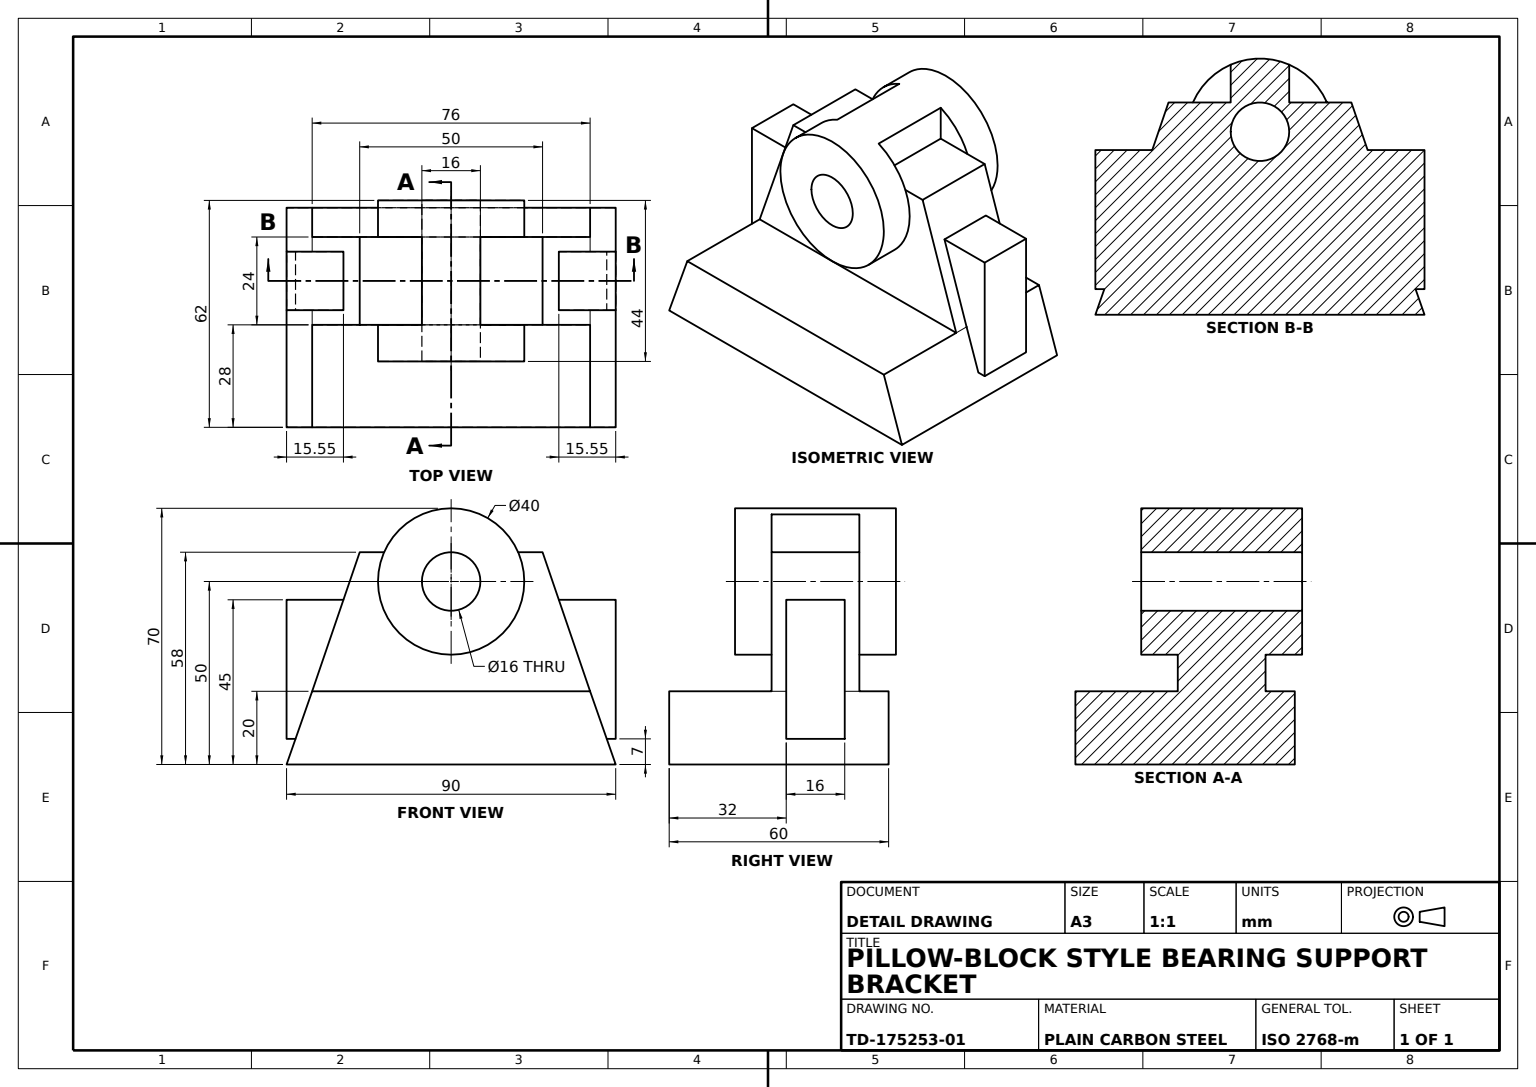
SolidWorks part; units mm, degrees
material "Plain Carbon Steel"
ref_plane "Front Plane" through (0, 0, 0) normal (0, 0, 1) x (1, 0, 0)
ref_plane "Top Plane" through (0, 0, 0) normal (0, 1, 0) x (1, 0, 0)
ref_plane "Right Plane" through (0, 0, 0) normal (1, 0, 0) x (0, 0, -1)
sketch "Base Profile Sketch" plane through (0, 0, 0) normal (0, 1, 0) x (1, 0, 0)
  line L1 (30, 0) -> (30, 45)
  line L2 (30, 45) -> (-30, 45)
  line L3 (-30, 45) -> (-30, -45)
  line L4 (-30, -45) -> (30, -45)
  line L5 (30, -45) -> (30, 0)
  dimension "D1" = 60
  dimension "D2" = 90
  dimension "D3" = 30
extrude "Base Block" add sketch "Base Profile Sketch" along normal blind 20
sketch "Base Recess Sketch" plane through (30, 0, 0) normal (1, 0, 0) x (0, 0, -1)
  line L1 (-45, 20) -> (45, 20) construction
  line L2 (38, 20) -> (45, 0)
  line L4 (-38, 20) -> (-45, 0)
  line L5 (-45, 0) -> (-45, 20)
  line L6 (-45, 20) -> (-38, 20)
  line L7 (45, 0) -> (45, 20)
  line L8 (45, 20) -> (38, 20)
  dimension "D1" = 7
extrude "Base Recess Cut" cut sketch "Base Recess Sketch" against normal blind 75
ref_plane "Hub Plane" through (12, 0, 0) normal (1, 0, 0) x (0, 0, -1)
ref_plane "Web Plane" through (2, 0, 0) normal (1, 0, 0) x (0, 0, -1)
sketch "Hub Circle Sketch" plane through (12, 0, 0) normal (1, 0, 0) x (0, 0, -1)
  circle A0 centre (0, 50) radius 20
  dimension "D1" = 40
  dimension "D2" = 50
extrude "Bearing Hub" add sketch "Hub Circle Sketch" against normal blind 44 separate body
sketch "Support Web Sketch" plane through (2, 0, 0) normal (1, 0, 0) x (0, 0, -1)
  line L0 (25, 20) -> (-25, 20)
  line L1 (-38, 20) -> (38, 20) construction
  line L3 (-25, 58) -> (-18.3303, 58)
  line L4 (-38, 20) -> (-25, 58)
  line L5 (-38, 20) -> (-25, 20)
  line L7 (38, 20) -> (25, 20)
  line L8 (38, 20) -> (25, 58)
  line L9 (25, 58) -> (18.3303, 58)
  circle A0 centre (0, 50) radius 20 construction
  arc A1 (-18.3303, 58) -> (18.3303, 58) centre (0, 50) ccw
  dimension "D1" = 13
  dimension "D2" = 19.6697
extrude "Support Web" add sketch "Support Web Sketch" against normal blind 24
ref_plane "Top Offset Plane" through (0, 70, 0) normal (0, 1, 0) x (1, 0, 0)
sketch "Side Window Sketch" plane through (2, 0, 0) normal (1, 0, 0) x (0, 0, -1)
  line L1 (-8, 68.3303) -> (-8, 58)
  line L2 (-18.3303, 58) -> (-8, 58)
  arc A1 (-8, 68.3303) -> (-18.3303, 58) centre (0, 50) ccw
extrude "Side Window Cut" cut sketch "Side Window Sketch" against normal blind 24
mirror "Side Window Mirror" about plane through (0, 0, 0) normal (0, 0, 1) of "Side Window Cut"
sketch "Bearing Bore Sketch" plane through (12, 0, 0) normal (1, 0, 0) x (0, 0, -1)
  circle A0 centre (0, 50) radius 8
  dimension "D1" = 16
extrude "Bearing Bore" cut sketch "Bearing Bore Sketch" against normal blind 57
ref_plane "Rib Plane" through (0, 0, 45) normal (0, 0, 1) x (1, 0, 0)
sketch "Side Rib Sketch" plane through (0, 0, 45) normal (0, 0, 1) x (1, 0, 0)
  line L2 (-10, 7) -> (-2, 7)
  line L3 (-2, 7) -> (-2, 45)
  line L4 (-2, 45) -> (-18, 45)
  line L5 (-18, 45) -> (-18, 7)
  line L6 (-18, 7) -> (-10, 7)
  dimension "D1" = 16
  dimension "D2" = 38
  dimension "D3" = 10
  dimension "D4" = 7
extrude "Side Rib" add sketch "Side Rib Sketch" against normal blind 20
mirror "Side Rib Mirror" about plane through (0, 0, 0) normal (0, 0, 1) of "Side Rib"
